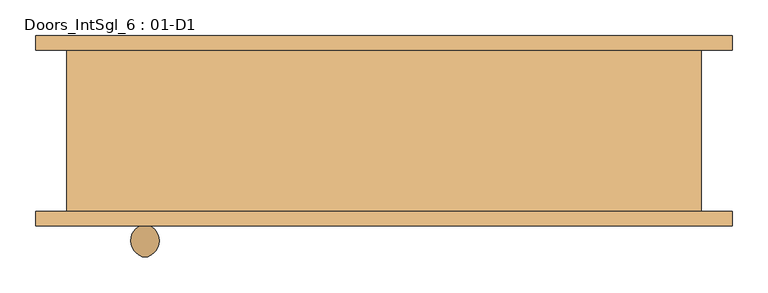
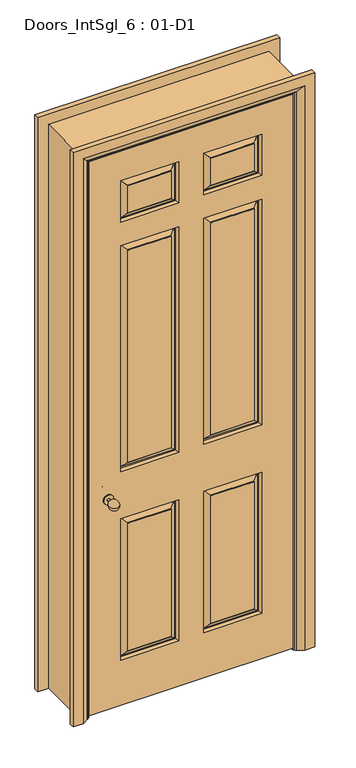
"""IFC4 building model written with IfcOpenShell, lengths in millimetres: door geometry, Doors_IntSgl_6 : 01-D1."""

from ifc_helpers import new_model, si_unit, point, frame, origin, place, context, project, spatial, polyline, circle_curve, ellipse_curve, trimmed, outline, extrude, faceted_brep, source, transform, mapped, element, save
from ifc_brep_helpers import plane_surface, cylinder_surface, revolved_surface, advanced_brep


def doors_intsgl_6_01_d1_21fcec07(model_context):
    return source(origin(), model_context, "Body", "SolidModel", [
        advanced_brep(
        [(-328.0, -55.5, 900.0), (-338.0, -55.5, 900.0), (-333.0, -11.062589, 900.0), (-328.0, -70.5, 900.0), (-338.0, -70.5, 900.0), (-353.0, -74.5, 900.0), (-313.0, -74.5, 900.0), (-353.0, -70.5, 900.0), (-313.0, -70.5, 900.0)],
        [
            (0, 1, circle_curve(frame((-333.0, -55.5, 900.0), z_axis=(0.0, 1.0, 0.0), x_axis=(-1.0, 0.0, 0.0)), 5.0)),
            (1, 2, circle_curve(frame((-329.8115138, -33.9213505, 900.0), z_axis=(0.0, 0.0, -1.0), x_axis=(0.0, -1.0, 0.0)), 23.0800654)),
            (2, 0, circle_curve(frame((-336.1884862, -33.9213505, 900.0), z_axis=(0.0, 0.0, -1.0), x_axis=(0.0, -1.0, 0.0)), 23.0800654)),
            (1, 0, circle_curve(frame((-333.0, -55.5, 900.0), z_axis=(0.0, 1.0, 0.0), x_axis=(-1.0, 0.0, 0.0)), 5.0)),
            (0, 3),
            (3, 4, circle_curve(frame((-333.0, -70.5, 900.0), z_axis=(0.0, 1.0, 0.0), x_axis=(-1.0, 0.0, 0.0)), 5.0)),
            (4, 1),
            (4, 3, circle_curve(frame((-333.0, -70.5, 900.0), z_axis=(0.0, 1.0, 0.0), x_axis=(-1.0, 0.0, 0.0)), 5.0)),
            (5, 6, circle_curve(frame((-333.0, -74.5, 900.0), z_axis=(0.0, -1.0, 0.0), x_axis=(1.0, 0.0, 0.0)), 20.0)),
            (6, 5, circle_curve(frame((-333.0, -74.5, 900.0), z_axis=(0.0, -1.0, 0.0), x_axis=(1.0, 0.0, 0.0)), 20.0)),
            (7, 8, circle_curve(frame((-333.0, -70.5, 900.0), z_axis=(0.0, 1.0, 0.0), x_axis=(1.0, 0.0, 0.0)), 20.0)),
            (8, 7, circle_curve(frame((-333.0, -70.5, 900.0), z_axis=(0.0, 1.0, 0.0), x_axis=(1.0, 0.0, 0.0)), 20.0)),
            (5, 7),
            (8, 6),
        ],
        [
            revolved_surface(trimmed(ellipse_curve(frame((-329.8115138, -33.9213505, 900.0), z_axis=(0.0, 0.0, 1.0), x_axis=(0.0, -1.0, 0.0)), 23.0800654, 23.0800654), [point((-333.0, -11.062589, 900.0))], [point((-338.0, -55.5, 900.0))], True, "CARTESIAN"), (-333.0, -70.5, 900.0), (0.0, -1.0, 0.0)),
            cylinder_surface(frame((-333.0, -70.5, 900.0), z_axis=(0.0, -1.0, 0.0), x_axis=(-1.0, 0.0, 0.0)), 5.0),
            plane_surface(frame((-313.0, -74.5, 900.0), z_axis=(0.0, -1.0, 0.0), x_axis=(0.0, 0.0, 1.0))),
            plane_surface(frame((-313.0, -70.5, 900.0), z_axis=(0.0, 1.0, 0.0), x_axis=(0.0, 0.0, -1.0))),
            cylinder_surface(frame((-333.0, -70.5, 900.0), z_axis=(0.0, -1.0, 0.0), x_axis=(1.0, 0.0, 0.0)), 20.0),
        ],
        [
            (0, [[1, 2, 3]]),
            (0, [[-2, 4, -3]]),
            (1, [[-1, 5, 6, 7]]),
            (1, [[-4, -7, 8, -5]]),
            (2, [[9, 10]]),
            (3, [[11, 12], [-6, -8]]),
            (4, [[-9, 13, -12, 14]]),
            (4, [[-10, -14, -11, -13]]),
        ],
    ),
        advanced_brep(
        [(-328.0, -131.5, 900.0), (-333.0, -175.937411, 900.0), (-338.0, -131.5, 900.0), (-338.0, -116.5, 900.0), (-328.0, -116.5, 900.0), (-353.0, -112.5, 900.0), (-313.0, -112.5, 900.0), (-353.0, -116.5, 900.0), (-313.0, -116.5, 900.0)],
        [
            (0, 1, circle_curve(frame((-336.1884862, -153.0786495, 900.0), z_axis=(0.0, 0.0, -1.0), x_axis=(0.0, 1.0, 0.0)), 23.0800654)),
            (1, 2, circle_curve(frame((-329.8115138, -153.0786495, 900.0), z_axis=(0.0, 0.0, -1.0), x_axis=(0.0, 1.0, 0.0)), 23.0800654)),
            (2, 0, circle_curve(frame((-333.0, -131.5, 900.0), z_axis=(0.0, -1.0, 0.0), x_axis=(-1.0, 0.0, 0.0)), 5.0)),
            (0, 2, circle_curve(frame((-333.0, -131.5, 900.0), z_axis=(0.0, -1.0, 0.0), x_axis=(-1.0, 0.0, 0.0)), 5.0)),
            (2, 3),
            (3, 4, circle_curve(frame((-333.0, -116.5, 900.0), z_axis=(0.0, -1.0, 0.0), x_axis=(-1.0, 0.0, 0.0)), 5.0)),
            (4, 0),
            (4, 3, circle_curve(frame((-333.0, -116.5, 900.0), z_axis=(0.0, -1.0, 0.0), x_axis=(-1.0, 0.0, 0.0)), 5.0)),
            (5, 6, circle_curve(frame((-333.0, -112.5, 900.0), z_axis=(0.0, 1.0, 0.0), x_axis=(1.0, 0.0, 0.0)), 20.0)),
            (6, 5, circle_curve(frame((-333.0, -112.5, 900.0), z_axis=(0.0, 1.0, 0.0), x_axis=(1.0, 0.0, 0.0)), 20.0)),
            (7, 8, circle_curve(frame((-333.0, -116.5, 900.0), z_axis=(0.0, -1.0, 0.0), x_axis=(1.0, 0.0, 0.0)), 20.0)),
            (8, 7, circle_curve(frame((-333.0, -116.5, 900.0), z_axis=(0.0, -1.0, 0.0), x_axis=(1.0, 0.0, 0.0)), 20.0)),
            (6, 8),
            (7, 5),
        ],
        [
            revolved_surface(trimmed(ellipse_curve(frame((-329.8115138, -153.0786495, 900.0), z_axis=(0.0, 0.0, -1.0), x_axis=(0.0, 1.0, 0.0)), 23.0800654, 23.0800654), [point((-333.0, -175.937411, 900.0))], [point((-338.0, -131.5, 900.0))], True, "CARTESIAN"), (-333.0, -116.5, 900.0), (0.0, 1.0, 0.0)),
            cylinder_surface(frame((-333.0, -116.5, 900.0), z_axis=(0.0, 1.0, 0.0), x_axis=(-1.0, 0.0, 0.0)), 5.0),
            plane_surface(frame((-313.0, -112.5, 900.0), z_axis=(0.0, 1.0, 0.0), x_axis=(0.0, 0.0, 1.0))),
            plane_surface(frame((-313.0, -116.5, 900.0), z_axis=(0.0, -1.0, 0.0), x_axis=(0.0, 0.0, -1.0))),
            cylinder_surface(frame((-333.0, -116.5, 900.0), z_axis=(0.0, 1.0, 0.0), x_axis=(1.0, 0.0, 0.0)), 20.0),
        ],
        [
            (0, [[1, 2, 3]]),
            (0, [[-1, 4, -2]]),
            (1, [[5, 6, 7, -3]]),
            (1, [[-7, 8, -5, -4]]),
            (2, [[9, 10]]),
            (3, [[11, 12], [-8, -6]]),
            (4, [[13, -11, 14, -10]]),
            (4, [[-14, -12, -13, -9]]),
        ],
    ),
        faceted_brep([(-408.0, -74.5, 2358.0), (408.0, -74.5, 2358.0), (408.0, -74.5, 8.0), (-408.0, -74.5, 8.0), (-50.0, -74.5, 800.0), (-283.0, -74.5, 800.0), (-283.0, -74.5, 200.0), (-50.0, -74.5, 200.0), (283.0, -74.5, 800.0), (50.0, -74.5, 800.0), (50.0, -74.5, 200.0), (283.0, -74.5, 200.0), (-50.0, -74.5, 1958.0), (-283.0, -74.5, 1958.0), (-283.0, -74.5, 1000.0), (-50.0, -74.5, 1000.0), (283.0, -74.5, 1958.0), (50.0, -74.5, 1958.0), (50.0, -74.5, 1000.0), (283.0, -74.5, 1000.0), (-50.0, -74.5, 2233.0), (-283.0, -74.5, 2233.0), (-283.0, -74.5, 2058.0), (-50.0, -74.5, 2058.0), (283.0, -74.5, 2233.0), (50.0, -74.5, 2233.0), (50.0, -74.5, 2058.0), (283.0, -74.5, 2058.0), (-80.0, -74.5, 230.0), (-253.0, -74.5, 230.0), (-253.0, -74.5, 770.0), (-80.0, -74.5, 770.0), (253.0, -74.5, 230.0), (80.0, -74.5, 230.0), (80.0, -74.5, 770.0), (253.0, -74.5, 770.0), (-80.0, -74.5, 1030.0), (-253.0, -74.5, 1030.0), (-253.0, -74.5, 1928.0), (-80.0, -74.5, 1928.0), (253.0, -74.5, 1030.0), (80.0, -74.5, 1030.0), (80.0, -74.5, 1928.0), (253.0, -74.5, 1928.0), (-80.0, -74.5, 2088.0), (-253.0, -74.5, 2088.0), (-253.0, -74.5, 2203.0), (-80.0, -74.5, 2203.0), (253.0, -74.5, 2088.0), (80.0, -74.5, 2088.0), (80.0, -74.5, 2203.0), (253.0, -74.5, 2203.0), (-408.0, -112.5, 2358.0), (-408.0, -112.5, 8.0), (408.0, -112.5, 8.0), (408.0, -112.5, 2358.0), (50.0, -112.5, 800.0), (283.0, -112.5, 800.0), (283.0, -112.5, 200.0), (50.0, -112.5, 200.0), (-283.0, -112.5, 800.0), (-50.0, -112.5, 800.0), (-50.0, -112.5, 200.0), (-283.0, -112.5, 200.0), (50.0, -112.5, 1958.0), (283.0, -112.5, 1958.0), (283.0, -112.5, 1000.0), (50.0, -112.5, 1000.0), (-283.0, -112.5, 1958.0), (-50.0, -112.5, 1958.0), (-50.0, -112.5, 1000.0), (-283.0, -112.5, 1000.0), (50.0, -112.5, 2233.0), (283.0, -112.5, 2233.0), (283.0, -112.5, 2058.0), (50.0, -112.5, 2058.0), (-283.0, -112.5, 2233.0), (-50.0, -112.5, 2233.0), (-50.0, -112.5, 2058.0), (-283.0, -112.5, 2058.0), (80.0, -112.5, 230.0), (253.0, -112.5, 230.0), (253.0, -112.5, 770.0), (80.0, -112.5, 770.0), (-253.0, -112.5, 230.0), (-80.0, -112.5, 230.0), (-80.0, -112.5, 770.0), (-253.0, -112.5, 770.0), (80.0, -112.5, 1030.0), (253.0, -112.5, 1030.0), (253.0, -112.5, 1928.0), (80.0, -112.5, 1928.0), (-253.0, -112.5, 1030.0), (-80.0, -112.5, 1030.0), (-80.0, -112.5, 1928.0), (-253.0, -112.5, 1928.0), (80.0, -112.5, 2088.0), (253.0, -112.5, 2088.0), (253.0, -112.5, 2203.0), (80.0, -112.5, 2203.0), (-253.0, -112.5, 2088.0), (-80.0, -112.5, 2088.0), (-80.0, -112.5, 2203.0), (-253.0, -112.5, 2203.0), (80.0, -111.5, 230.0), (80.0, -111.5, 770.0), (58.0, -97.5, 208.0), (78.0, -111.5, 228.0), (78.0, -111.5, 772.0), (58.0, -97.5, 792.0), (53.0, -97.5, 203.0), (53.0, -97.5, 797.0), (253.0, -111.5, 770.0), (255.0, -111.5, 772.0), (275.0, -97.5, 792.0), (280.0, -97.5, 797.0), (253.0, -111.5, 230.0), (255.0, -111.5, 228.0), (275.0, -97.5, 208.0), (280.0, -97.5, 203.0), (-253.0, -111.5, 230.0), (-253.0, -111.5, 770.0), (-275.0, -97.5, 208.0), (-255.0, -111.5, 228.0), (-255.0, -111.5, 772.0), (-275.0, -97.5, 792.0), (-280.0, -97.5, 203.0), (-280.0, -97.5, 797.0), (-80.0, -111.5, 770.0), (-78.0, -111.5, 772.0), (-58.0, -97.5, 792.0), (-53.0, -97.5, 797.0), (-80.0, -111.5, 230.0), (-78.0, -111.5, 228.0), (-58.0, -97.5, 208.0), (-53.0, -97.5, 203.0), (80.0, -111.5, 1030.0), (80.0, -111.5, 1928.0), (58.0, -97.5, 1008.0), (78.0, -111.5, 1028.0), (78.0, -111.5, 1930.0), (58.0, -97.5, 1950.0), (53.0, -97.5, 1003.0), (53.0, -97.5, 1955.0), (253.0, -111.5, 1928.0), (255.0, -111.5, 1930.0), (275.0, -97.5, 1950.0), (280.0, -97.5, 1955.0), (253.0, -111.5, 1030.0), (255.0, -111.5, 1028.0), (275.0, -97.5, 1008.0), (280.0, -97.5, 1003.0), (-253.0, -111.5, 1030.0), (-253.0, -111.5, 1928.0), (-275.0, -97.5, 1008.0), (-255.0, -111.5, 1028.0), (-255.0, -111.5, 1930.0), (-275.0, -97.5, 1950.0), (-280.0, -97.5, 1003.0), (-280.0, -97.5, 1955.0), (-80.0, -111.5, 1928.0), (-78.0, -111.5, 1930.0), (-58.0, -97.5, 1950.0), (-53.0, -97.5, 1955.0), (-80.0, -111.5, 1030.0), (-78.0, -111.5, 1028.0), (-58.0, -97.5, 1008.0), (-53.0, -97.5, 1003.0), (80.0, -111.5, 2088.0), (80.0, -111.5, 2203.0), (58.0, -97.5, 2066.0), (78.0, -111.5, 2086.0), (78.0, -111.5, 2205.0), (58.0, -97.5, 2225.0), (53.0, -97.5, 2061.0), (53.0, -97.5, 2230.0), (253.0, -111.5, 2203.0), (255.0, -111.5, 2205.0), (275.0, -97.5, 2225.0), (280.0, -97.5, 2230.0), (253.0, -111.5, 2088.0), (255.0, -111.5, 2086.0), (275.0, -97.5, 2066.0), (280.0, -97.5, 2061.0), (-253.0, -111.5, 2088.0), (-253.0, -111.5, 2203.0), (-275.0, -97.5, 2066.0), (-255.0, -111.5, 2086.0), (-255.0, -111.5, 2205.0), (-275.0, -97.5, 2225.0), (-280.0, -97.5, 2061.0), (-280.0, -97.5, 2230.0), (-80.0, -111.5, 2203.0), (-78.0, -111.5, 2205.0), (-58.0, -97.5, 2225.0), (-53.0, -97.5, 2230.0), (-80.0, -111.5, 2088.0), (-78.0, -111.5, 2086.0), (-58.0, -97.5, 2066.0), (-53.0, -97.5, 2061.0), (-80.0, -75.5, 230.0), (-80.0, -75.5, 770.0), (-58.0, -89.5, 208.0), (-78.0, -75.5, 228.0), (-78.0, -75.5, 772.0), (-58.0, -89.5, 792.0), (-53.0, -89.5, 203.0), (-53.0, -89.5, 797.0), (-253.0, -75.5, 770.0), (-255.0, -75.5, 772.0), (-275.0, -89.5, 792.0), (-280.0, -89.5, 797.0), (-253.0, -75.5, 230.0), (-255.0, -75.5, 228.0), (-275.0, -89.5, 208.0), (-280.0, -89.5, 203.0), (253.0, -75.5, 230.0), (253.0, -75.5, 770.0), (275.0, -89.5, 208.0), (255.0, -75.5, 228.0), (255.0, -75.5, 772.0), (275.0, -89.5, 792.0), (280.0, -89.5, 203.0), (280.0, -89.5, 797.0), (80.0, -75.5, 770.0), (78.0, -75.5, 772.0), (58.0, -89.5, 792.0), (53.0, -89.5, 797.0), (80.0, -75.5, 230.0), (78.0, -75.5, 228.0), (58.0, -89.5, 208.0), (53.0, -89.5, 203.0), (-80.0, -75.5, 1030.0), (-80.0, -75.5, 1928.0), (-58.0, -89.5, 1008.0), (-78.0, -75.5, 1028.0), (-78.0, -75.5, 1930.0), (-58.0, -89.5, 1950.0), (-53.0, -89.5, 1003.0), (-53.0, -89.5, 1955.0), (-253.0, -75.5, 1928.0), (-255.0, -75.5, 1930.0), (-275.0, -89.5, 1950.0), (-280.0, -89.5, 1955.0), (-253.0, -75.5, 1030.0), (-255.0, -75.5, 1028.0), (-275.0, -89.5, 1008.0), (-280.0, -89.5, 1003.0), (253.0, -75.5, 1030.0), (253.0, -75.5, 1928.0), (275.0, -89.5, 1008.0), (255.0, -75.5, 1028.0), (255.0, -75.5, 1930.0), (275.0, -89.5, 1950.0), (280.0, -89.5, 1003.0), (280.0, -89.5, 1955.0), (80.0, -75.5, 1928.0), (78.0, -75.5, 1930.0), (58.0, -89.5, 1950.0), (53.0, -89.5, 1955.0), (80.0, -75.5, 1030.0), (78.0, -75.5, 1028.0), (58.0, -89.5, 1008.0), (53.0, -89.5, 1003.0), (-80.0, -75.5, 2088.0), (-80.0, -75.5, 2203.0), (-58.0, -89.5, 2066.0), (-78.0, -75.5, 2086.0), (-78.0, -75.5, 2205.0), (-58.0, -89.5, 2225.0), (-53.0, -89.5, 2061.0), (-53.0, -89.5, 2230.0), (-253.0, -75.5, 2203.0), (-255.0, -75.5, 2205.0), (-275.0, -89.5, 2225.0), (-280.0, -89.5, 2230.0), (-253.0, -75.5, 2088.0), (-255.0, -75.5, 2086.0), (-275.0, -89.5, 2066.0), (-280.0, -89.5, 2061.0), (253.0, -75.5, 2088.0), (253.0, -75.5, 2203.0), (275.0, -89.5, 2066.0), (255.0, -75.5, 2086.0), (255.0, -75.5, 2205.0), (275.0, -89.5, 2225.0), (280.0, -89.5, 2061.0), (280.0, -89.5, 2230.0), (80.0, -75.5, 2203.0), (78.0, -75.5, 2205.0), (58.0, -89.5, 2225.0), (53.0, -89.5, 2230.0), (80.0, -75.5, 2088.0), (78.0, -75.5, 2086.0), (58.0, -89.5, 2066.0), (53.0, -89.5, 2061.0)], [[[0, 1, 2, 3], [4, 5, 6, 7], [8, 9, 10, 11], [12, 13, 14, 15], [16, 17, 18, 19], [20, 21, 22, 23], [24, 25, 26, 27]], [[28, 29, 30, 31]], [[32, 33, 34, 35]], [[36, 37, 38, 39]], [[40, 41, 42, 43]], [[44, 45, 46, 47]], [[48, 49, 50, 51]], [[52, 53, 54, 55], [56, 57, 58, 59], [60, 61, 62, 63], [64, 65, 66, 67], [68, 69, 70, 71], [72, 73, 74, 75], [76, 77, 78, 79]], [[80, 81, 82, 83]], [[84, 85, 86, 87]], [[88, 89, 90, 91]], [[92, 93, 94, 95]], [[96, 97, 98, 99]], [[100, 101, 102, 103]], [[3, 53, 52, 0]], [[2, 54, 53, 3]], [[1, 55, 54, 2]], [[0, 52, 55, 1]], [[104, 80, 83, 105]], [[106, 107, 108, 109]], [[56, 59, 110, 111]], [[83, 82, 112, 105]], [[108, 113, 114, 109]], [[111, 115, 57, 56]], [[82, 81, 116, 112]], [[113, 117, 118, 114]], [[115, 119, 58, 57]], [[104, 116, 81, 80]], [[107, 117, 113, 108], [105, 112, 116, 104]], [[106, 118, 117, 107]], [[110, 119, 115, 111], [109, 114, 118, 106]], [[59, 58, 119, 110]], [[120, 84, 87, 121]], [[122, 123, 124, 125]], [[60, 63, 126, 127]], [[87, 86, 128, 121]], [[124, 129, 130, 125]], [[127, 131, 61, 60]], [[86, 85, 132, 128]], [[129, 133, 134, 130]], [[131, 135, 62, 61]], [[120, 132, 85, 84]], [[123, 133, 129, 124], [121, 128, 132, 120]], [[122, 134, 133, 123]], [[126, 135, 131, 127], [125, 130, 134, 122]], [[63, 62, 135, 126]], [[136, 88, 91, 137]], [[138, 139, 140, 141]], [[64, 67, 142, 143]], [[91, 90, 144, 137]], [[140, 145, 146, 141]], [[143, 147, 65, 64]], [[90, 89, 148, 144]], [[145, 149, 150, 146]], [[147, 151, 66, 65]], [[136, 148, 89, 88]], [[139, 149, 145, 140], [137, 144, 148, 136]], [[138, 150, 149, 139]], [[142, 151, 147, 143], [141, 146, 150, 138]], [[67, 66, 151, 142]], [[152, 92, 95, 153]], [[154, 155, 156, 157]], [[68, 71, 158, 159]], [[95, 94, 160, 153]], [[156, 161, 162, 157]], [[159, 163, 69, 68]], [[94, 93, 164, 160]], [[161, 165, 166, 162]], [[163, 167, 70, 69]], [[152, 164, 93, 92]], [[155, 165, 161, 156], [153, 160, 164, 152]], [[154, 166, 165, 155]], [[158, 167, 163, 159], [157, 162, 166, 154]], [[71, 70, 167, 158]], [[168, 96, 99, 169]], [[170, 171, 172, 173]], [[72, 75, 174, 175]], [[99, 98, 176, 169]], [[172, 177, 178, 173]], [[175, 179, 73, 72]], [[98, 97, 180, 176]], [[177, 181, 182, 178]], [[179, 183, 74, 73]], [[168, 180, 97, 96]], [[171, 181, 177, 172], [169, 176, 180, 168]], [[170, 182, 181, 171]], [[174, 183, 179, 175], [173, 178, 182, 170]], [[75, 74, 183, 174]], [[184, 100, 103, 185]], [[186, 187, 188, 189]], [[76, 79, 190, 191]], [[103, 102, 192, 185]], [[188, 193, 194, 189]], [[191, 195, 77, 76]], [[102, 101, 196, 192]], [[193, 197, 198, 194]], [[195, 199, 78, 77]], [[184, 196, 101, 100]], [[187, 197, 193, 188], [185, 192, 196, 184]], [[186, 198, 197, 187]], [[190, 199, 195, 191], [189, 194, 198, 186]], [[79, 78, 199, 190]], [[200, 28, 31, 201]], [[202, 203, 204, 205]], [[4, 7, 206, 207]], [[31, 30, 208, 201]], [[204, 209, 210, 205]], [[207, 211, 5, 4]], [[30, 29, 212, 208]], [[209, 213, 214, 210]], [[211, 215, 6, 5]], [[200, 212, 29, 28]], [[203, 213, 209, 204], [201, 208, 212, 200]], [[202, 214, 213, 203]], [[206, 215, 211, 207], [205, 210, 214, 202]], [[7, 6, 215, 206]], [[216, 32, 35, 217]], [[218, 219, 220, 221]], [[8, 11, 222, 223]], [[35, 34, 224, 217]], [[220, 225, 226, 221]], [[223, 227, 9, 8]], [[34, 33, 228, 224]], [[225, 229, 230, 226]], [[227, 231, 10, 9]], [[216, 228, 33, 32]], [[219, 229, 225, 220], [217, 224, 228, 216]], [[218, 230, 229, 219]], [[222, 231, 227, 223], [221, 226, 230, 218]], [[11, 10, 231, 222]], [[232, 36, 39, 233]], [[234, 235, 236, 237]], [[12, 15, 238, 239]], [[39, 38, 240, 233]], [[236, 241, 242, 237]], [[239, 243, 13, 12]], [[38, 37, 244, 240]], [[241, 245, 246, 242]], [[243, 247, 14, 13]], [[232, 244, 37, 36]], [[235, 245, 241, 236], [233, 240, 244, 232]], [[234, 246, 245, 235]], [[238, 247, 243, 239], [237, 242, 246, 234]], [[15, 14, 247, 238]], [[248, 40, 43, 249]], [[250, 251, 252, 253]], [[16, 19, 254, 255]], [[43, 42, 256, 249]], [[252, 257, 258, 253]], [[255, 259, 17, 16]], [[42, 41, 260, 256]], [[257, 261, 262, 258]], [[259, 263, 18, 17]], [[248, 260, 41, 40]], [[251, 261, 257, 252], [249, 256, 260, 248]], [[250, 262, 261, 251]], [[254, 263, 259, 255], [253, 258, 262, 250]], [[19, 18, 263, 254]], [[264, 44, 47, 265]], [[266, 267, 268, 269]], [[20, 23, 270, 271]], [[47, 46, 272, 265]], [[268, 273, 274, 269]], [[271, 275, 21, 20]], [[46, 45, 276, 272]], [[273, 277, 278, 274]], [[275, 279, 22, 21]], [[264, 276, 45, 44]], [[267, 277, 273, 268], [265, 272, 276, 264]], [[266, 278, 277, 267]], [[270, 279, 275, 271], [269, 274, 278, 266]], [[23, 22, 279, 270]], [[280, 48, 51, 281]], [[282, 283, 284, 285]], [[24, 27, 286, 287]], [[51, 50, 288, 281]], [[284, 289, 290, 285]], [[287, 291, 25, 24]], [[50, 49, 292, 288]], [[289, 293, 294, 290]], [[291, 295, 26, 25]], [[280, 292, 49, 48]], [[283, 293, 289, 284], [281, 288, 292, 280]], [[282, 294, 293, 283]], [[286, 295, 291, 287], [285, 290, 294, 282]], [[27, 26, 295, 286]]]),
        faceted_brep([(-410.0, -112.5, 0.0), (-442.0, -112.5, 0.0), (-442.0, 112.5, 0.0), (-410.0, 112.5, 0.0), (-410.0, 112.5, 2360.0), (-410.0, -112.5, 2360.0), (-442.0, 112.5, 2392.0), (-442.0, -112.5, 2392.0), (410.0, -112.5, 0.0), (410.0, 112.5, 0.0), (442.0, 112.5, 0.0), (442.0, -112.5, 0.0), (410.0, -112.5, 2360.0), (442.0, -112.5, 2392.0), (442.0, 112.5, 2392.0), (410.0, 112.5, 2360.0)], [[[0, 1, 2, 3]], [[3, 4, 5, 0]], [[2, 6, 4, 3]], [[1, 7, 6, 2]], [[0, 5, 7, 1]], [[8, 9, 10, 11]], [[12, 8, 11, 13]], [[13, 11, 10, 14]], [[14, 10, 9, 15]], [[15, 9, 8, 12]], [[4, 15, 12, 5]], [[6, 14, 15, 4]], [[7, 13, 14, 6]], [[5, 12, 13, 7]]]),
        extrude(outline(polyline([(0.0, -391.0), (2341.0, -391.0), (2341.0, 391.0), (0.0, 391.0), (0.0, 410.0), (2360.0, 410.0), (2360.0, -410.0), (0.0, -410.0), (0.0, -391.0)])), frame((0.0, -72.5, 0.0), z_axis=(0.0, 1.0, 0.0), x_axis=(0.0, 0.0, 1.0)), (0.0, 0.0, 1.0), 32.0),
        advanced_brep(
        [(-485.0, 132.5, 0.0), (-445.0, 132.5, 0.0), (-419.0, 118.5, 0.0), (-415.0, 112.5, 0.0), (-485.0, 112.5, 0.0), (-485.0, 112.5, 2435.0), (-485.0, 132.5, 2435.0), (-415.0, 112.5, 2365.0), (415.0, 112.5, 2365.0), (415.0, 112.5, 0.0), (485.0, 112.5, 0.0), (485.0, 112.5, 2435.0), (-419.0, 118.5, 2369.0), (-445.0, 132.5, 2395.0), (485.0, 132.5, 2435.0), (485.0, 132.5, 0.0), (445.0, 132.5, 0.0), (445.0, 132.5, 2395.0), (419.0, 118.5, 0.0), (419.0, 118.5, 2369.0)],
        [
            (0, 1),
            (1, 2),
            (2, 3, circle_curve(frame((-423.0, 111.5, 0.0), z_axis=(0.0, 0.0, -1.0), x_axis=(-1.0, 0.0, 0.0)), 8.0622577)),
            (3, 4),
            (4, 0),
            (4, 5),
            (5, 6),
            (6, 0),
            (3, 7),
            (7, 8),
            (8, 9),
            (9, 10),
            (10, 11),
            (11, 5),
            (2, 12),
            (12, 7, ellipse_curve(frame((-423.0, 111.5, 2373.0), z_axis=(-0.7071067811865475, 0.0, -0.7071067811865475), x_axis=(0.7071067811865474, 0.0, -0.7071067811865476)), 11.4017543, 8.0622577)),
            (1, 13),
            (13, 12),
            (6, 14),
            (14, 15),
            (15, 16),
            (16, 17),
            (17, 13),
            (10, 15),
            (14, 11),
            (9, 18, circle_curve(frame((423.0, 111.5, 0.0), z_axis=(0.0, 0.0, -1.0), x_axis=(1.0, 0.0, 0.0)), 8.0622577)),
            (18, 16),
            (19, 18),
            (8, 19, ellipse_curve(frame((423.0, 111.5, 2373.0), z_axis=(0.7071067811865475, 0.0, -0.7071067811865475), x_axis=(0.7071067811865474, 0.0, 0.7071067811865476)), 11.4017543, 8.0622577)),
            (19, 17),
            (12, 19),
        ],
        [
            plane_surface(frame((-415.0, 112.5, 0.0), z_axis=(0.0, 0.0, -1.0), x_axis=(0.0, 1.0, 0.0))),
            plane_surface(frame((-485.0, 132.5, 0.0), z_axis=(-1.0, 0.0, 0.0), x_axis=(0.0, 0.0, 1.0))),
            plane_surface(frame((-485.0, 112.5, 0.0), z_axis=(0.0, -1.0, 0.0), x_axis=(0.0, 0.0, 1.0))),
            cylinder_surface(frame((-423.0, 111.5, 0.0), z_axis=(0.0, 0.0, -1.0), x_axis=(-1.0, 0.0, 0.0)), 8.0622577),
            plane_surface(frame((-419.0, 118.5, 0.0), z_axis=(0.4740998230350183, 0.8804710999221749, 0.0), x_axis=(0.0, 0.0, 1.0))),
            plane_surface(frame((-445.0, 132.5, 0.0), z_axis=(0.0, 1.0, 0.0), x_axis=(0.0, 0.0, 1.0))),
            plane_surface(frame((485.0, 132.5, 2435.0), z_axis=(1.0, 0.0, 0.0), x_axis=(0.0, 0.0, -1.0))),
            plane_surface(frame((415.0, 112.5, 0.0), z_axis=(0.0, 0.0, -1.0), x_axis=(0.0, 1.0, 0.0))),
            cylinder_surface(frame((423.0, 111.5, 2365.0), z_axis=(0.0, 0.0, 1.0), x_axis=(1.0, 0.0, 0.0)), 8.0622577),
            plane_surface(frame((419.0, 118.5, 2369.0), z_axis=(-0.4740998230350183, 0.8804710999221749, 0.0), x_axis=(0.0, 0.0, -1.0))),
            plane_surface(frame((-485.0, 132.5, 2435.0), z_axis=(0.0, 0.0, 1.0), x_axis=(1.0, 0.0, 0.0))),
            cylinder_surface(frame((-415.0, 111.5, 2373.0), z_axis=(-1.0, 0.0, 0.0), x_axis=(0.0, 0.0, 1.0)), 8.0622577),
            plane_surface(frame((-419.0, 118.5, 2369.0), z_axis=(0.0, 0.8804710999221749, -0.4740998230350183), x_axis=(1.0, 0.0, 0.0))),
        ],
        [
            (0, [[1, 2, 3, 4, 5]]),
            (1, [[6, 7, 8, -5]]),
            (2, [[9, 10, 11, 12, 13, 14, -6, -4]]),
            (3, [[15, 16, -9, -3]]),
            (4, [[17, 18, -15, -2]]),
            (5, [[-8, 19, 20, 21, 22, 23, -17, -1]]),
            (6, [[-13, 24, -20, 25]]),
            (7, [[-24, -12, 26, 27, -21]]),
            (8, [[28, -26, -11, 29]]),
            (9, [[-22, -27, -28, 30]]),
            (10, [[-14, -25, -19, -7]]),
            (11, [[31, -29, -10, -16]]),
            (12, [[-23, -30, -31, -18]]),
        ],
    ),
        advanced_brep(
        [(485.0, -132.5, 0.0), (445.0, -132.5, 0.0), (419.0, -118.5, 0.0), (415.0, -112.5, 0.0), (485.0, -112.5, 0.0), (485.0, -112.5, 2435.0), (485.0, -132.5, 2435.0), (415.0, -112.5, 2365.0), (-415.0, -112.5, 2365.0), (-415.0, -112.5, 0.0), (-485.0, -112.5, 0.0), (-485.0, -112.5, 2435.0), (419.0, -118.5, 2369.0), (445.0, -132.5, 2395.0), (-485.0, -132.5, 2435.0), (-485.0, -132.5, 0.0), (-445.0, -132.5, 0.0), (-445.0, -132.5, 2395.0), (-419.0, -118.5, 0.0), (-419.0, -118.5, 2369.0)],
        [
            (0, 1),
            (1, 2),
            (2, 3, circle_curve(frame((423.0, -111.5, 0.0), z_axis=(0.0, 0.0, -1.0), x_axis=(1.0, 0.0, 0.0)), 8.0622577)),
            (3, 4),
            (4, 0),
            (4, 5),
            (5, 6),
            (6, 0),
            (3, 7),
            (7, 8),
            (8, 9),
            (9, 10),
            (10, 11),
            (11, 5),
            (2, 12),
            (12, 7, ellipse_curve(frame((423.0, -111.5, 2373.0), z_axis=(0.7071067811865475, 0.0, -0.7071067811865475), x_axis=(-0.7071067811865474, 0.0, -0.7071067811865476)), 11.4017543, 8.0622577)),
            (1, 13),
            (13, 12),
            (6, 14),
            (14, 15),
            (15, 16),
            (16, 17),
            (17, 13),
            (10, 15),
            (14, 11),
            (9, 18, circle_curve(frame((-423.0, -111.5, 0.0), z_axis=(0.0, 0.0, -1.0), x_axis=(-1.0, 0.0, 0.0)), 8.0622577)),
            (18, 16),
            (19, 18),
            (8, 19, ellipse_curve(frame((-423.0, -111.5, 2373.0), z_axis=(-0.7071067811865475, 0.0, -0.7071067811865475), x_axis=(-0.7071067811865474, 0.0, 0.7071067811865476)), 11.4017543, 8.0622577)),
            (19, 17),
            (12, 19),
        ],
        [
            plane_surface(frame((415.0, -112.5, 0.0), z_axis=(0.0, 0.0, -1.0), x_axis=(0.0, -1.0, 0.0))),
            plane_surface(frame((485.0, -132.5, 0.0), z_axis=(1.0, 0.0, 0.0), x_axis=(0.0, 0.0, 1.0))),
            plane_surface(frame((485.0, -112.5, 0.0), z_axis=(0.0, 1.0, 0.0), x_axis=(0.0, 0.0, 1.0))),
            cylinder_surface(frame((423.0, -111.5, 0.0), z_axis=(0.0, 0.0, -1.0), x_axis=(1.0, 0.0, 0.0)), 8.0622577),
            plane_surface(frame((419.0, -118.5, 0.0), z_axis=(-0.4740998230350183, -0.8804710999221749, 0.0), x_axis=(0.0, 0.0, 1.0))),
            plane_surface(frame((445.0, -132.5, 0.0), z_axis=(0.0, -1.0, 0.0), x_axis=(0.0, 0.0, 1.0))),
            plane_surface(frame((-485.0, -132.5, 2435.0), z_axis=(-1.0, 0.0, 0.0), x_axis=(0.0, 0.0, -1.0))),
            plane_surface(frame((-415.0, -112.5, 0.0), z_axis=(0.0, 0.0, -1.0), x_axis=(0.0, -1.0, 0.0))),
            cylinder_surface(frame((-423.0, -111.5, 2365.0), z_axis=(0.0, 0.0, 1.0), x_axis=(-1.0, 0.0, 0.0)), 8.0622577),
            plane_surface(frame((-419.0, -118.5, 2369.0), z_axis=(0.4740998230350183, -0.8804710999221749, 0.0), x_axis=(0.0, 0.0, -1.0))),
            plane_surface(frame((485.0, -132.5, 2435.0), z_axis=(0.0, 0.0, 1.0), x_axis=(-1.0, 0.0, 0.0))),
            cylinder_surface(frame((415.0, -111.5, 2373.0), z_axis=(1.0, 0.0, 0.0), x_axis=(0.0, 0.0, 1.0)), 8.0622577),
            plane_surface(frame((419.0, -118.5, 2369.0), z_axis=(0.0, -0.8804710999221749, -0.4740998230350183), x_axis=(-1.0, 0.0, 0.0))),
        ],
        [
            (0, [[1, 2, 3, 4, 5]]),
            (1, [[6, 7, 8, -5]]),
            (2, [[9, 10, 11, 12, 13, 14, -6, -4]]),
            (3, [[15, 16, -9, -3]]),
            (4, [[17, 18, -15, -2]]),
            (5, [[-8, 19, 20, 21, 22, 23, -17, -1]]),
            (6, [[-13, 24, -20, 25]]),
            (7, [[-24, -12, 26, 27, -21]]),
            (8, [[28, -26, -11, 29]]),
            (9, [[-22, -27, -28, 30]]),
            (10, [[-14, -25, -19, -7]]),
            (11, [[31, -29, -10, -16]]),
            (12, [[-23, -30, -31, -18]]),
        ],
    ),
    ])


if __name__ == "__main__":
    model = new_model("IFC4")
    model_context = context("Model", 3, world=origin())
    ifc_project = project(units=[si_unit("LENGTHUNIT", "METRE", prefix="MILLI")], contexts=[model_context])
    site = spatial("IfcSite", under=ifc_project)
    building = spatial("IfcBuilding", under=site)
    placement = place(None, origin())
    doors_intsgl_6_01_d1_shape = doors_intsgl_6_01_d1_21fcec07(model_context)
    element("IfcDoor", 1, ObjectType="Doors_IntSgl_6 : 01-D1", at=placement, inside=building, context=model_context, shape_type="MappedRepresentation", body=[
        mapped(doors_intsgl_6_01_d1_shape, transform((0.0, 0.0, 0.0), x_axis=(1.0, 0.0, 0.0), y_axis=(0.0, 1.0, 0.0), z_axis=(0.0, 0.0, 1.0))),
    ])
    save(model, "model.ifc")

# Revit data of these elements
# Type "Doors_IntSgl_6 : 01-D1"
#   Type Mark = "49"
#   Type Comments = "Internal Single"
#   Operation = "SingleSwingRight"
#   Construction Type Id = "MDOOR"
#   Manufacturer = "Revit"
#   Keynote = "L20"
#   Description = "Internal Single Door"
#   Analytic Construction = "Metal"
#   UnderCut = 8 mm
#   Tolerance = 2 mm
#   Thickness = 38 mm
#   Structural Tolerance = 8 mm
#   StopDepth = 32 mm
#   Stop Thickness = 19 mm
#   Stile Top Rail = 125 mm
#   Stile Shutting = 125 mm
#   Stile Muntin Rail = 100 mm
#   Stile Lock Rail = 200 mm
#   Stile Intermediate/Frieze = 100 mm
#   Stile Hanging = 125 mm
#   Stile Bottom Rail = 200 mm
#   Rough Width = 900 mm
#   Rough Height = 2400 mm
#   Height to Top Lock Rail = 1000 mm
#   Heat Transfer Coefficient (U) = 3.7021 W/(m²·K)
#   Handle Z Distance = 900 mm
#   Handle X Distance = 75 mm
#   Frame Thickness = 32 mm
#   Door Panel Width = 816 mm
#   Height = 2400 mm
#   Width = 900 mm
#   Door Panel Thickness = 38 mm
#   Door Panel Offset = 0 mm
#   Door Panel Height = 2350 mm
#   Architrave Setback = 5 mm
#   Vis - Ironmongery = yes
#   Define Thermal Properties by = 1
#   Material Ironmongery = Door - Handle
#   Material Frame = Door - Frame/Mullion
#   Material Door = Door - Panel
#   Material Architrave = Door - Architrave
#   Visual Light Transmittance = 0
#   Solar Heat Gain Coefficient = 0
#   Function = (empty or 0)
#   Wall Closure = (empty or 0)
# Element 1 (IfcDoor, "Doors_IntSgl_6 : 01-D1")
#   Materials on its faces: "Door - Panel", "Door - Architrave", "Door - Frame/Mullion", "Door - Handle"
# Materials
#   "Door - Handle": colour RGB 247 247 247, transparency 0
#   "Door - Frame/Mullion": class "Wood", colour RGB 212 179 113, transparency 0
#   "Door - Panel": class "Wood", colour RGB 154 90 5, transparency 0
#   "Door - Architrave": class "Wood", colour RGB 154 90 5, transparency 0
